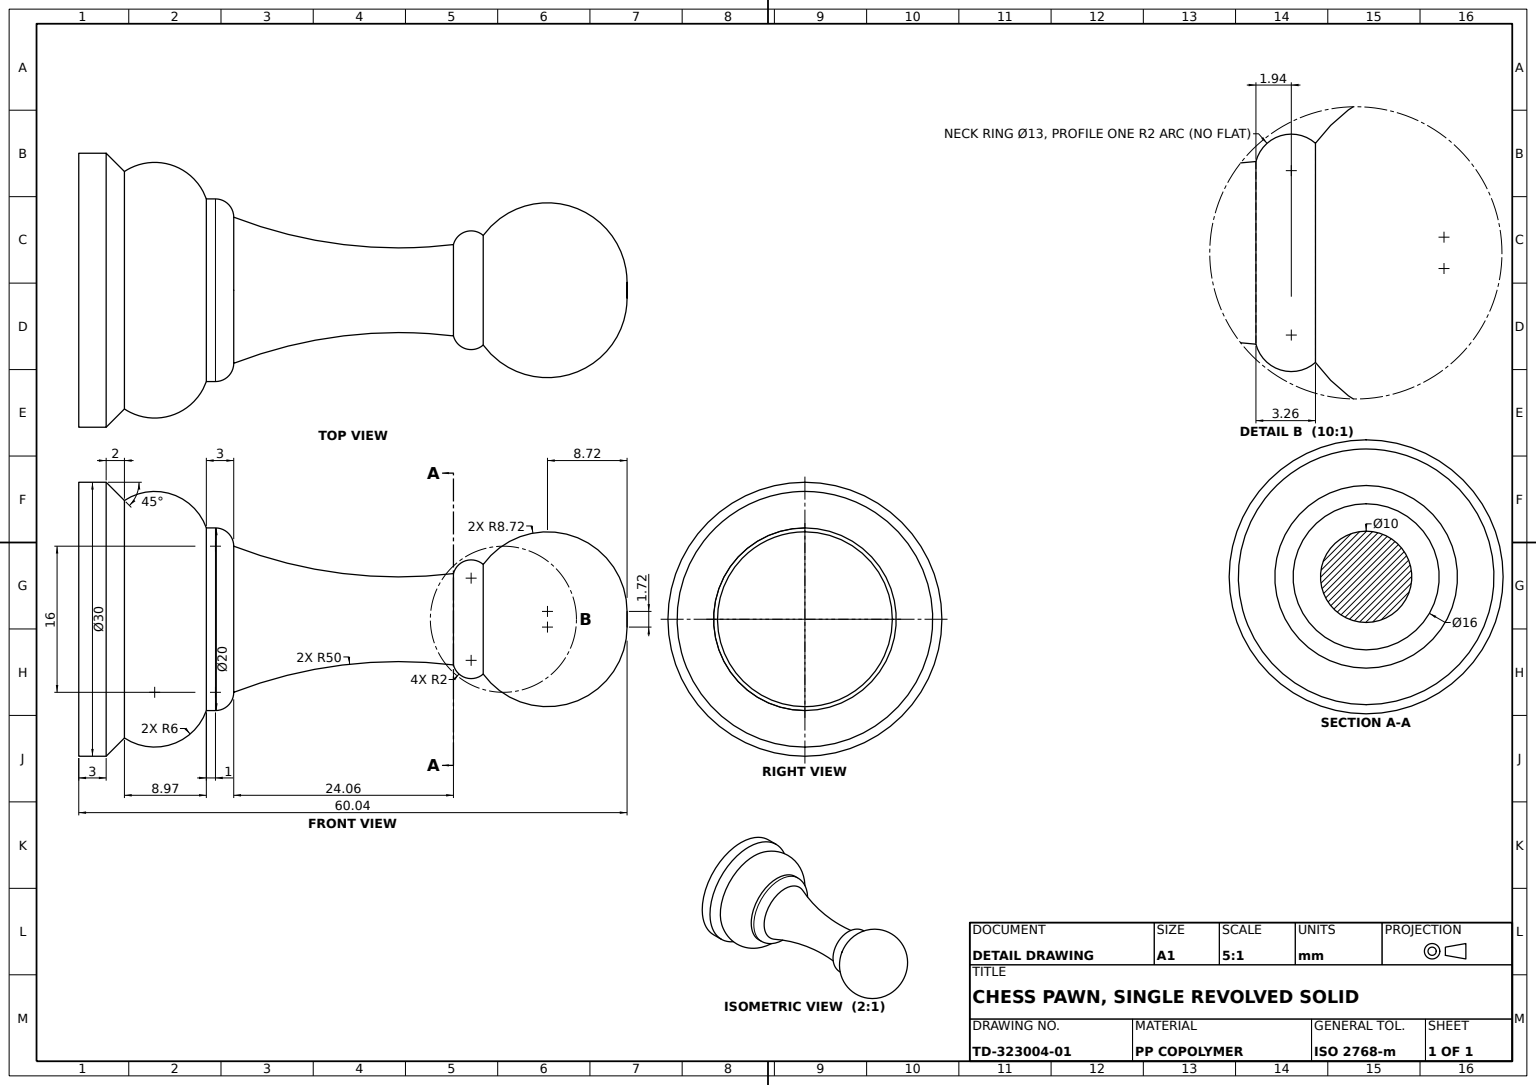
from build123d import *


with BuildPart() as part:
    # Pawn Profile Sketch → Pawn Body Revolve (revolve)
    with BuildSketch(Plane.XY, mode=Mode.PRIVATE) as pawn_body_revolve_sk:
        with BuildLine():
            Line((0, 0), (15, 0))
            Line((15, 0), (15, 3))
            Line((15, 3), (13, 5))
            ThreePointArc((13, 5), (13.688325627, 10.216881481), (10, 13.97))
            Line((10, 13.97), (10, 14.97))
            ThreePointArc((10, 14.97), (9.414213562, 16.384213562), (8, 16.97))
            ThreePointArc((8, 16.97), (5.019495729, 28.81539847), (5, 41.03))
            ThreePointArc((5, 41.03), (6.412519214, 42.380086131), (6, 44.29))
            ThreePointArc((6, 44.29), (9, 54.436534055), (0, 60))
            Line((0, 60), (0, 0))
        make_face()
    revolve(pawn_body_revolve_sk.sketch.rotate(Axis((0, 0, 0), (0, 1, 0)), 90), axis=Axis((0, 0, 0), (0, 1, 0)))


solid = part.part
